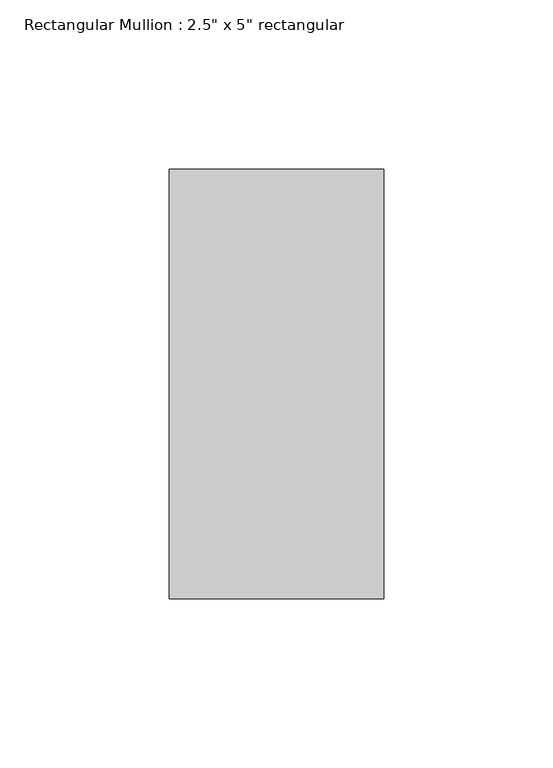
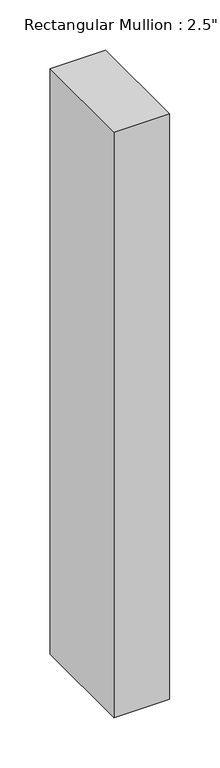
"""IFC4 building model written with IfcOpenShell, lengths in millimetres: member geometry."""

from ifc_helpers import new_model, si_unit, frame, origin, place, context, project, spatial, polyline, outline, extrude, source, transform, mapped, element, save


def member_3301b6a7(model_context):
    return source(origin(), model_context, "Body", "SweptSolid", [
        extrude(outline(polyline([(31.75, 63.5), (31.75, -63.5), (-31.75, -63.5), (-31.75, 63.5), (31.75, 63.5)])), frame((0.0, 0.0, -709.0542001), z_axis=(0.0, 0.0, 1.0), x_axis=(1.0, 0.0, 0.0)), (0.0, 0.0, 1.0), 709.0542001),
    ])


if __name__ == "__main__":
    model = new_model("IFC4")
    model_context = context("Model", 3, world=origin())
    ifc_project = project(units=[si_unit("LENGTHUNIT", "METRE", prefix="MILLI")], contexts=[model_context])
    site = spatial("IfcSite", under=ifc_project)
    building = spatial("IfcBuilding", under=site)
    placement = place(None, origin())
    member_shape = member_3301b6a7(model_context)
    element("IfcMember", 1, ObjectType="Rectangular Mullion : 2.5\" x 5\" rectangular", at=placement, inside=building, context=model_context, shape_type="MappedRepresentation", body=[
        mapped(member_shape, transform((0.0, 0.0, 0.0), x_axis=(1.0, 0.0, 0.0), y_axis=(0.0, 1.0, 0.0), z_axis=(0.0, 0.0, 1.0))),
    ])
    save(model, "model.ifc")

# Revit data of these elements
# Type "Rectangular Mullion : 2.5\" x 5\" rectangular"
#   built-in parameter 1007304 = 0.416667 (stored number, unit not read)
#   built-in parameter 1007301 = 0.104167 (stored number, unit not read)
#   built-in parameter 1007300 = 0.104167 (stored number, unit not read)
# Element 1 (IfcMember, "Rectangular Mullion : 2.5\" x 5\" rectangular")
#   Materials on its faces: "Aluminum"
# Materials
#   "Aluminum": class "Metal", colour RGB 247 247 247, transparency 0, Description = "Aluminum 6061", Cost = 0
